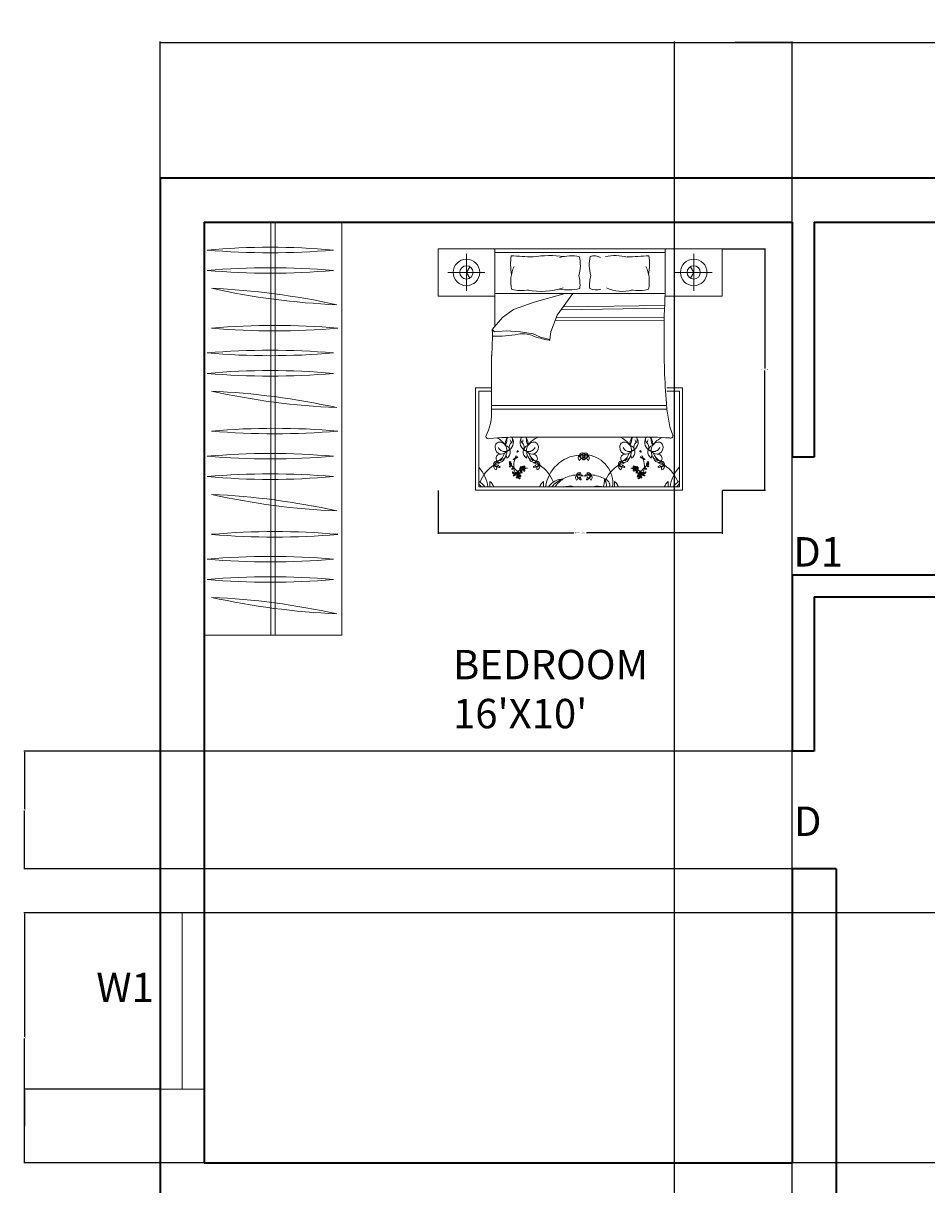
# Model space of a CAD drawing. Units: inches. Extents: x -4347 to -3836, y 955 to 1521.
# Tile 9 of 11: x -4347 to -4162, y 1284 to 1521. Entities that reach past the tile are written whole.
import ezdxf

# ---------------------------------------------------------------- set-up
doc = ezdxf.new("R2010")
doc.units = ezdxf.units.IN
doc.header["$MEASUREMENT"] = 0
for name, color, linetype, lineweight in [('A-ANNO-DIMS', 2, 'Continuous', 18), ('A-ANNO-TEXT', 7, 'Continuous', 18), ('A-AREA-IDEN', 7, 'Continuous', 18), ('A-FURN', 8, 'Continuous', 13), ('A-GLAZ', 4, 'Continuous', 18), ('A-WALL', 7, 'Continuous', 35)]:
    doc.layers.add(name, color=color, linetype=linetype, lineweight=lineweight)
doc.styles.get("Standard").update_dxf_attribs({"font": 'arial.ttf'})
doc.dimstyles.get("Standard").update_dxf_attribs({"dimtxt": 0.18, "dimasz": 0.18, "dimexe": 0.18, "dimexo": 0.0625, "dimgap": 0.09, "dimtad": 0, "dimtih": 1, "dimtoh": 1, "dimdec": 0, "dimzin": 0, "dimdsep": 46, "dimlunit": 3, "dimtxsty": 'Standard', "dimcen": 0.09, "dimadec": 0, "dimazin": 0, "dimtfac": 1, "dimtdec": 0, "dimtofl": 0, "dimtmove": 0, "dimatfit": 3, "dimfxl": 1, "dimtolj": 1, "dimtzin": 0, "dimarcsym": 0})

# ---------------------------------------------------------------- blocks, each defined once
blk = doc.blocks.new('*D1')
at = {"layer": 'A-ANNO-DIMS', "color": 0, "lineweight": -2, "transparency": 16777216}
for p, q in [((-4318.58, 1489.85), (-4318.58, 1517.61)), ((-4318.4, 1517.43), (-4135.47, 1517.43)), ((-3931.76, 1517.43), (-4114.69, 1517.43)), ((-3931.58, 1489.85), (-3931.58, 1517.61))]:
    blk.add_line(p, q, dxfattribs=at)
at = {"layer": 'A-ANNO-DIMS', "color": 0, "transparency": 16777216}
for points in [[(-4318.4, 1517.46), (-4318.4, 1517.4), (-4318.58, 1517.43)], [(-3931.76, 1517.46), (-3931.76, 1517.4), (-3931.58, 1517.43)]]:
    blk.add_solid(points, dxfattribs=at)
at = {"layer": 'Defpoints', "color": 0, "transparency": 16777216}
for p in [(-3931.58, 1517.43), (-4318.58, 1489.79), (-3931.58, 1489.79)]:
    blk.add_point(p, dxfattribs=at)
at = {"layer": 'A-ANNO-DIMS', "color": 0, "transparency": 16777216, "insert": (-4125.08, 1517.43), "char_height": 6, "attachment_point": 5}
blk.add_mtext('\\A1;32\'-3"', dxfattribs=at)
blk = doc.blocks.new('BED-DOUBLE-WITH-NIGHTSTANDS')
for p, q in [((0, 49.3), (57.97, 49.3)), ((5.8, 40.68), (5.8, 48.26)), ((11.59, 49.3), (11.59, 33.39)), ((46.38, 48.56), (11.59, 48.56)), ((52.18, 40.68), (52.18, 48.26)), ((9.59, 44.47), (2.01, 44.47)), ((48.39, 44.47), (55.96, 44.47)), ((11.59, 40.14), (46.38, 40.14)), ((15.42, 36.89), (19.65, 38.42)), ((19.65, 38.42), (25.97, 40.14)), ((27.52, 40.14), (24.34, 35.72)), ((13.19, 35.25), (15.42, 36.89)), ((24.34, 35.72), (23.05, 32.32)), ((46.2, 37.14), (25.15, 36.84)), ((46.22, 37.73), (25.58, 37.44)), ((11.08, 32.79), (13.19, 35.25)), ((46.17, 34.72), (23.93, 34.63)), ((46.17, 35.31), (24.16, 35.23)), ((11.55, 32.32), (11.08, 32.79)), ((13.89, 32.55), (11.55, 32.32)), ((16.83, 32.32), (13.89, 32.55)), ((19.41, 31.96), (16.83, 32.32)), ((20.94, 31.26), (19.41, 31.96)), ((22.82, 30.79), (20.94, 31.26)), ((23.05, 32.32), (22.82, 30.79)), ((7.65, 20.88), (10.93, 20.88)), ((7.65, 0), (7.65, 20.88)), ((10.93, 20.21), (8.32, 20.21)), ((8.32, 20.21), (8.32, 0.67)), ((49.25, 20.21), (46.69, 20.21)), ((46.7, 20.88), (49.92, 20.88)), ((49.25, 0.67), (49.25, 20.21)), ((49.92, 20.88), (49.92, 0)), ((46.64, 17.27), (10.93, 17.27)), ((46.7, 16.54), (10.93, 16.54)), ((40.76, 10.85), (17.22, 10.85)), ((14.04, 6.55), (13.91, 7.2)), ((18.09, 6.55), (18.22, 7.2)), ((39.48, 6.55), (39.35, 7.2)), ((43.53, 6.55), (43.66, 7.2)), ((8.32, 0.67), (49.25, 0.67)), ((49.92, 0), (7.65, 0))]:
    blk.add_line(p, q)
for points in [[(11.59, 39.64), (0, 39.64), (0, 49.3)], [(46.38, 49.3), (46.38, 39.64), (57.97, 39.64), (57.97, 49.3)], [(5.8, 44.47), (6.47, 45.64)], [(52.18, 44.47), (51.5, 45.64)], [(5.8, 44.47), (6.47, 43.3)], [(52.18, 44.47), (51.5, 43.3)]]:
    blk.add_lwpolyline(points)
for points in [[(14.92, 47.86, 0.074897), (15, 44.07, -0.472817)], [(28.72, 43.86, 0.14099), (28.83, 47.72, 0.235245)], [(31.19, 43.86, -0.14099), (31.08, 47.72, -0.235245)], [(43.05, 47.86, -0.074897), (42.98, 44.07, 0.472817)], [(10.95, 27.48, 0.001242), (10.93, 16.48, -0.127202), (9.76, 10.99)], [(46.63, 17.72, 0.056112), (47.05, 14.53, 0.095341), (47.86, 11.46)]]:
    blk.add_lwpolyline(points, format="xyb")
for centre, radius in [((5.8, 44.47), 2.71), ((5.8, 44.47), 1.35), ((52.18, 44.47), 2.71), ((52.18, 44.47), 1.35), ((16.42, 2.89), 0.148), ((17.39, 4.45), 0.148), ((40.18, 4.45), 0.148), ((41.15, 2.89), 0.148)]:
    blk.add_circle(centre, radius)
for centre, radius, start, end in [((46.88, 599.58), 552.65, 266.6852, 267.1498), ((22.87, 26.88), 21.03, 82.2196, 99.497), ((27.31, 37.51), 10.33, 81.5249, 103.96), ((31.87, 44.97), 2.87, 63.3437, 106.1026), ((36.17, 37.71), 10.19, 76.3427, 101.1841), ((11.09, 599.58), 552.65, 272.8502, 273.3148), ((22.31, 42.55), 7.47, 155.1316, 191.7583), ((35.66, 42.55), 7.47, 348.2417, 24.8684), ((21.88, 41.92), 7.1, 354.0129, 15.8293), ((38.03, 41.92), 7.1, 164.1707, 185.9871), ((16.99, 48.54), 7.77, 255.1039, 281.0369), ((21.08, 54.06), 13.48, 258.0397, 289.2615), ((26.54, 51.12), 10.22, 259.8617, 283.6238), ((32.26, 43.97), 3.07, 245.0183, 288.5407), ((37.63, 47.96), 7.38, 243.8761, 286.1746), ((40.98, 48.54), 7.77, 258.9631, 284.8961), ((150.31, 33.06), 104.17, 176.1, 180.9282), ((-42.08, 31.34), 53.18, 355.8294, 1.553), ((12.07, 53.32), 21.88, 267.4519, 281.3392), ((17.3, 27.24), 4.72, 66.2616, 101.3392), ((26.84, 52.7), 22.48, 250.1194, 259.3383), ((182.02, 29.27), 135.88, 179.1145, 184.8735), ((22.69, 30.74), 0.14, 268.8623, 19.7536), ((10.3, 11.03), 0.535, 183.98, 297.3412), ((16.53, -49.5), 60.35, 89.3433, 95.6887), ((12.63, 8.87), 0.979, 84.4856, 181.0538), ((10.07, 6.77), 4.39, 33.6671, 63.2997), ((12.33, 8.15), 1.74, 355.2933, 76.921), ((15.95, 9.38), 2.24, 145.785, 184.7304), ((11.68, 10.42), 2.4, 328.8218, 9.1554), ((14.66, 10.21), 0.698, 120.0293, 142.325), ((13.54, 9.8), 1.85, 289.2822, 29.1751), ((15.73, 8.81), 1.19, 131.5653, 195.1471), ((13.26, 9.46), 1.67, 7.436, 29.9149), ((14.36, 10.35), 0.867, 311.5653, 23.8354), ((14.66, 10.21), 0.698, 44.4517, 63.558), ((18.58, 9.8), 1.85, 150.8249, 250.7178), ((17.76, 10.35), 0.867, 156.1646, 228.4347), ((17.47, 10.21), 0.698, 113.229, 135.5483), ((16.4, 8.81), 1.19, 344.8529, 48.4347), ((18.86, 9.46), 1.67, 150.0851, 172.564), ((17.47, 10.21), 0.698, 37.675, 66.7144), ((16.17, 9.38), 2.24, 355.2696, 34.215), ((20.44, 10.42), 2.4, 169.7133, 211.1782), ((19.8, 8.15), 1.74, 103.079, 184.7067), ((22.05, 6.77), 4.39, 111.4941, 146.3329), ((19.5, 8.87), 0.979, 358.9462, 95.5144), ((38.07, 8.87), 0.979, 84.4856, 181.0538), ((35.52, 6.77), 4.39, 33.6671, 68.5059), ((37.77, 8.15), 1.74, 355.2933, 76.921), ((41.4, 9.38), 2.24, 145.785, 184.7304), ((37.13, 10.42), 2.4, 328.8218, 10.2867), ((40.1, 10.21), 0.698, 113.2856, 142.325), ((38.99, 9.8), 1.85, 289.2822, 29.1751), ((41.17, 8.81), 1.19, 131.5653, 195.1471), ((38.71, 9.46), 1.67, 7.436, 29.9149), ((40.1, 10.21), 0.698, 44.4517, 66.7144), ((39.81, 10.35), 0.867, 311.5653, 23.8354), ((42.53, -45.54), 56.41, 85.2402, 91.8035), ((44.03, 9.8), 1.85, 150.8249, 250.7178), ((43.21, 10.35), 0.867, 156.1646, 228.4347), ((42.91, 10.21), 0.698, 106.6343, 135.5483), ((41.84, 8.81), 1.19, 344.8529, 48.4347), ((44.31, 9.46), 1.67, 150.0851, 172.564), ((42.91, 10.21), 0.698, 37.675, 72.5814), ((41.62, 9.38), 2.24, 355.2696, 34.215), ((45.89, 10.42), 2.4, 169.249, 211.1782), ((45.24, 8.15), 1.74, 103.079, 184.7067), ((47.5, 6.77), 4.39, 113.6453, 146.3329), ((44.94, 8.87), 0.979, 358.9462, 95.5144), ((47.42, 11.17), 0.528, 246.5219, 33.8264), ((13.03, 8.73), 1.39, 174.9449, 262.8857), ((12.71, 6.5), 0.87, 80.264, 250.8688), ((13.57, 9.26), 1.35, 201.5819, 291.4221), ((10.99, 8.42), 2.74, 301.2614, 341.7045), ((12.79, 9.04), 1.68, 272.3591, 324.0401), ((10.96, 8.2), 3.11, 326.2883, 356.5076), ((13.32, 7.8), 1.44, 299.9085, 73.1337), ((15.95, 9.38), 2.24, 212.7011, 216.3445), ((14.23, 8.4), 0.36, 257.3041, 15.1471), ((20.25, 4.94), 4.8, 153.0032, 159.8941), ((16.23, 7.86), 0.112, 102.7051, 280.4384), ((16.22, 7.93), 0.182, 280.4384, 100.4136), ((18.81, 7.8), 1.44, 106.8663, 240.0915), ((17.89, 8.4), 0.36, 164.8529, 282.6959), ((16.17, 9.38), 2.24, 323.6555, 327.2989), ((19.34, 9.04), 1.68, 215.9599, 267.6409), ((18.55, 9.26), 1.35, 248.5779, 338.4181), ((21.17, 8.2), 3.11, 183.4924, 213.7117), ((21.14, 8.42), 2.74, 198.2955, 238.7386), ((19.1, 8.73), 1.39, 277.1143, 5.0551), ((19.41, 6.5), 0.87, 289.1312, 99.736), ((29.44, -0.35), 7.57, 94.4623, 172.255), ((29.47, 6.63), 0.84, 137.7873, 219.1145), ((28.52, 6.66), 0.632, 298.5391, 58.3627), ((29.45, 7.02), 0.628, 63.0274, 163.8037), ((28.82, 8.49), 1.29, 271.4585, 315.3727), ((29.34, 6.11), 1.2, 45.5411, 114.3101), ((30.43, 12.25), 5.3, 252.593, 267.2582), ((29.47, 7.17), 0.619, 177.7585, 283.852), ((30.66, 7.82), 1.91, 198.9159, 238.011), ((30.16, 6.11), 1.2, 65.6899, 134.4589), ((29.07, 12.25), 5.3, 272.7418, 287.407), ((30.05, 7.02), 0.628, 16.1963, 116.9726), ((30.69, 8.49), 1.29, 224.6273, 268.5415), ((28.84, 7.82), 1.91, 301.989, 341.0841), ((30.03, 7.17), 0.619, 256.148, 2.2415), ((30.99, 6.66), 0.632, 121.6373, 241.4609), ((30.03, 6.63), 0.84, 320.8855, 42.2127), ((29.82, 1.4), 5.86, 352.8636, 81.8197), ((38.47, 8.73), 1.39, 174.9449, 262.8857), ((38.16, 6.5), 0.87, 80.264, 250.8688), ((39.02, 9.26), 1.35, 201.5819, 291.4221), ((36.43, 8.42), 2.74, 301.2614, 341.7045), ((38.23, 9.04), 1.68, 272.3591, 324.0401), ((36.4, 8.2), 3.11, 326.2883, 356.5076), ((38.76, 7.8), 1.44, 299.9085, 73.1337), ((41.4, 9.38), 2.24, 212.7011, 216.3445), ((39.68, 8.4), 0.36, 257.3041, 15.1471), ((41.35, 7.93), 0.182, 79.5864, 259.5616), ((41.34, 7.86), 0.112, 259.5616, 77.2949), ((37.32, 4.94), 4.8, 20.1059, 26.9968), ((44.25, 7.8), 1.44, 106.8663, 240.0915), ((43.34, 8.4), 0.36, 164.8529, 282.6959), ((41.62, 9.38), 2.24, 323.6555, 327.2989), ((44.78, 9.04), 1.68, 215.9599, 267.6409), ((44, 9.26), 1.35, 248.5779, 338.4181), ((46.61, 8.2), 3.11, 183.4924, 213.7117), ((46.58, 8.42), 2.74, 198.2955, 238.7386), ((44.54, 8.73), 1.39, 277.1143, 5.0551), ((44.86, 6.5), 0.87, 289.1312, 99.736), ((15.64, -1.1), 7.57, 124.3865, 158.5908), ((12.18, 4.97), 0.84, 167.7115, 249.0387), ((11.97, 5.3), 0.628, 92.9516, 193.728), ((10.69, 6.25), 1.29, 301.3827, 345.2969), ((12.34, 4.45), 1.2, 75.4653, 144.2343), ((10.22, 10.32), 5.3, 282.5173, 297.1824), ((11.35, 4.52), 0.632, 328.4633, 88.2869), ((12.62, 6.59), 1.91, 228.8402, 267.9352), ((11.91, 5.44), 0.619, 207.6827, 313.7762), ((12.53, 5.56), 0.533, 63.9755, 143.2681), ((12.28, 5.05), 0.0819, 313.7762, 249.7183), ((12.5, 6.76), 1.09, 265.969, 344.3045), ((12.55, 4.82), 0.0457, 101.4834, 217.9409), ((12.56, 4.77), 0.094, 267.9352, 101.4834), ((13.67, 5.32), 1.16, 96.1662, 141.5825), ((14.73, 5.55), 0.246, 101.5637, 142.6358), ((14.52, 5.33), 0.148, 273.2768, 86.7232), ((14.73, 5.05), 0.244, 217.7621, 259.0403), ((14.7, 5.47), 0.141, 91.1081, 181.8675), ((14.99, 5.38), 0.448, 203.4276, 227.6104), ((14.53, 5.75), 0.355, 288.7263, 352.5032), ((14.85, 5.18), 0.305, 80.3487, 133.6538), ((14.79, 5.43), 0.242, 229.7889, 317.6792), ((14.52, 4.92), 0.343, 355.053, 68.3618), ((14.79, 4.86), 0.483, 83.0852, 105.7171), ((14.77, 5.73), 0.114, 345.2356, 144.9248), ((14.75, 4.9), 0.113, 232.4737, 355.053), ((11.44, 0.86), 5.5, 43.1541, 52.0459), ((14.88, 5.36), 0.127, 317.6792, 80.3487), ((15.59, 6.13), 0.304, 101.3256, 154.4621), ((15.15, 7.16), 0.916, 280.2588, 300.656), ((15.36, 7.9), 1.63, 268.3264, 277.1302), ((20.25, 4.94), 4.8, 163.5842, 183.8277), ((14.95, 7.16), 0.931, 308.2101, 316.3071), ((15.52, 6.55), 0.278, 278.3432, 4.2869), ((15.37, 6.79), 0.486, 300.656, 332.6341), ((15.74, 6.47), 0.118, 55.7657, 157.4417), ((15.92, 6.58), 0.118, 84.3784, 186.0543), ((15.81, 7.06), 0.486, 269.1859, 301.164), ((15.95, 6.81), 0.278, 237.5332, 323.4768), ((15.68, 7.6), 0.931, 285.5129, 293.6099), ((15.59, 7.42), 0.916, 301.164, 321.5612), ((16.29, 6.55), 0.304, 87.3579, 140.4944), ((14.84, 7.58), 1.63, 324.6898, 333.4936), ((16.26, 4.67), 0.673, 304.5369, 16.3699), ((17.19, 4.48), 0.476, 127.3105, 187.9252), ((16.54, 4.53), 0.489, 355.0106, 41.658), ((17.22, 4.65), 0.201, 126.1046, 271.4281), ((17.2, 4.71), 0.145, 353.7526, 131.7054), ((17.59, 4.68), 0.246, 101.5637, 176.365), ((17.39, 4.87), 0.355, 288.7263, 352.5032), ((17.63, 4.85), 0.114, 345.2356, 144.9248), ((18.45, 5.32), 1.16, 38.4175, 83.8338), ((19.62, 6.76), 1.09, 195.6955, 274.031), ((19.59, 5.56), 0.533, 36.7319, 116.0245), ((19.57, 4.77), 0.094, 78.5166, 272.0648), ((19.79, 4.45), 1.2, 35.7657, 104.5347), ((21.91, 10.32), 5.3, 242.8176, 257.4827), ((19.5, 6.59), 1.91, 272.0648, 311.1598), ((19.58, 4.82), 0.0457, 322.0591, 78.5166), ((20.21, 5.44), 0.619, 226.2238, 332.3173), ((19.85, 5.08), 0.0494, 290.2667, 226.2271), ((20.78, 4.52), 0.632, 91.7131, 211.5367), ((20.15, 5.3), 0.628, 346.272, 87.0484), ((21.43, 6.25), 1.29, 194.7031, 238.6173), ((19.94, 4.97), 0.84, 290.9613, 12.2885), ((16.49, -1.1), 7.57, 21.4092, 55.6135), ((29.6, 6.65), 0.0819, 283.852, 219.9245), ((29.7, 6.28), 0.094, 238.011, 71.5592), ((29.71, 6.32), 0.0457, 71.5592, 188.0167), ((29.81, 6.28), 0.094, 108.4408, 301.989), ((29.79, 6.32), 0.0457, 351.9833, 108.4408), ((29.9, 6.68), 0.0494, 320.1909, 256.0209), ((41.08, -1.1), 7.57, 124.3865, 158.5908), ((37.42, 5.3), 0.628, 92.9516, 193.728), ((37.63, 4.97), 0.84, 167.7115, 249.0387), ((36.13, 6.25), 1.29, 301.3827, 345.2969), ((37.78, 4.45), 1.2, 75.4653, 144.2343), ((35.66, 10.32), 5.3, 282.5173, 297.1824), ((37.36, 5.44), 0.619, 207.6827, 313.7762), ((38.07, 6.59), 1.91, 228.8402, 267.9352), ((36.79, 4.52), 0.632, 328.4633, 88.2869), ((37.98, 5.56), 0.533, 63.9755, 143.2681), ((37.73, 5.05), 0.0819, 313.7762, 249.7183), ((37.95, 6.76), 1.09, 265.969, 344.3045), ((37.99, 4.82), 0.0457, 101.4834, 217.9409), ((38, 4.77), 0.094, 267.9352, 101.4834), ((39.12, 5.32), 1.16, 96.1662, 141.5825), ((39.94, 4.85), 0.114, 35.0752, 194.7644), ((40.18, 4.87), 0.355, 187.4968, 251.2737), ((39.98, 4.68), 0.246, 3.635, 78.4363), ((40.37, 4.71), 0.145, 48.2946, 186.2474), ((40.35, 4.65), 0.201, 268.5719, 53.8954), ((41.03, 4.53), 0.489, 138.342, 184.9894), ((41.31, 4.67), 0.673, 163.6301, 235.4631), ((40.38, 4.48), 0.476, 352.0748, 52.6895), ((41.98, 7.42), 0.916, 218.4388, 238.836), ((41.28, 6.55), 0.304, 39.5056, 92.6421), ((42.73, 7.58), 1.63, 206.5064, 215.3102), ((41.62, 6.81), 0.278, 216.5232, 302.4668), ((41.89, 7.6), 0.931, 246.3901, 254.4871), ((41.76, 7.06), 0.486, 238.836, 270.8141), ((41.65, 6.58), 0.118, 353.9457, 95.6216), ((41.83, 6.47), 0.118, 22.5583, 124.2343), ((42.05, 6.55), 0.278, 175.7131, 261.6568), ((42.2, 6.79), 0.486, 207.3659, 239.344), ((37.32, 4.94), 4.8, 356.1723, 16.4158), ((42.62, 7.16), 0.931, 223.6929, 231.7899), ((42.42, 7.16), 0.916, 239.344, 259.7412), ((42.21, 7.9), 1.63, 262.8698, 271.6736), ((41.98, 6.13), 0.304, 25.5379, 78.6744), ((46.13, 0.86), 5.5, 127.9541, 136.8459), ((42.69, 5.36), 0.127, 99.6513, 222.3208), ((42.78, 5.43), 0.242, 222.3208, 310.2111), ((42.72, 5.18), 0.305, 46.3462, 99.6513), ((42.8, 5.73), 0.114, 35.0752, 194.7644), ((43.04, 5.75), 0.355, 187.4968, 251.2737), ((43.05, 4.92), 0.343, 111.6382, 184.947), ((42.82, 4.9), 0.113, 184.947, 307.5263), ((42.78, 4.86), 0.483, 74.2829, 96.9148), ((42.87, 5.47), 0.141, 358.1325, 88.8919), ((42.58, 5.38), 0.448, 312.3896, 336.5724), ((42.84, 5.55), 0.246, 37.3642, 78.4363), ((42.84, 5.05), 0.244, 280.9597, 322.2379), ((43.05, 5.33), 0.148, 93.2768, 266.7232), ((45.07, 6.76), 1.09, 195.6955, 274.031), ((43.9, 5.32), 1.16, 38.4175, 83.8338), ((45.04, 5.56), 0.533, 36.7319, 116.0245), ((45.01, 4.77), 0.094, 78.5166, 272.0648), ((45.23, 4.45), 1.2, 35.7657, 104.5347), ((47.35, 10.32), 5.3, 242.8176, 257.4827), ((44.95, 6.59), 1.91, 272.0648, 311.1598), ((45.02, 4.82), 0.0457, 322.0591, 78.5166), ((45.66, 5.44), 0.619, 226.2238, 332.3173), ((45.29, 5.08), 0.0494, 290.2667, 226.2271), ((46.22, 4.52), 0.632, 91.7131, 211.5367), ((46.88, 6.25), 1.29, 194.7031, 238.6173), ((45.6, 5.3), 0.628, 346.272, 87.0484), ((45.39, 4.97), 0.84, 290.9613, 12.2885), ((41.93, -1.1), 7.57, 21.4092, 55.6135), ((2.69, -0.35), 7.57, 7.745, 41.8856), ((15.24, 4.18), 0.304, 101.3256, 154.4621), ((14.81, 5.21), 0.916, 280.2588, 300.656), ((15.02, 5.95), 1.63, 268.3264, 277.1302), ((14.61, 5.21), 0.931, 308.2101, 316.3071), ((15.35, 3.65), 0.165, 146.8636, 236.9021), ((17.67, 7.28), 4.31, 235.1882, 238.8844), ((15.63, 3.89), 0.446, 199.4799, 267.6828), ((15.18, 4.6), 0.278, 278.3432, 4.2869), ((15.58, 3.72), 0.384, 212.8155, 277.3992), ((15.03, 4.84), 0.486, 300.656, 332.6341), ((15.39, 4.52), 0.118, 55.7657, 157.4417), ((15.36, 3.46), 0.446, 266.9701, 338.2913), ((13, 6.64), 4.31, 302.6784, 306.3746), ((15.47, 3.11), 0.165, 214.3538, 304.3923), ((15.53, 3.73), 0.171, 238.8844, 314.2646), ((17.86, 4.82), 2.41, 184.756, 209.2041), ((21.32, 9.95), 7.92, 222.2412, 232.1744), ((15.49, 3.35), 0.384, 280.3057, 17.1958), ((15.46, 3.31), 0.171, 306.3746, 21.7548), ((15.74, 3.42), 0.129, 19.3605, 201.7548), ((15.74, 3.52), 0.129, 311.8703, 134.2646), ((18.16, 2.34), 2.57, 153.7819, 158.2913), ((16.11, 4.1), 0.673, 247.2305, 319.0635), ((15.89, 3.87), 0.396, 264.4544, 310.6188), ((17.86, 4.82), 2.41, 214.0033, 222.4917), ((16.18, 3.72), 0.409, 218.3208, 298.8162), ((18.1, 1.62), 2.89, 120.544, 139.818), ((16.11, 2.62), 0.146, 148.0499, 225.6268), ((16.38, 2.45), 0.465, 104.7558, 148.0499), ((16.12, 2.78), 0.291, 247.4086, 351.4386), ((16.26, 3.1), 0.201, 126.1046, 271.4281), ((16.24, 3.15), 0.145, 353.7526, 131.7054), ((16.46, 3.21), 0.476, 70.0041, 130.6188), ((16.2, 2.77), 0.0978, 262.906, 7.132), ((16.1, 2.98), 0.203, 0.0645, 61.1507), ((16.15, 3.15), 0.232, 311.8413, 355.7877), ((16.15, 3.79), 0.489, 297.7043, 344.3516), ((16.62, 3.12), 0.246, 101.5637, 176.365), ((16.62, 2.62), 0.244, 151.2196, 259.0403), ((16.59, 3.03), 0.141, 91.1081, 181.8675), ((16.88, 2.94), 0.448, 203.4276, 227.6104), ((16.74, 2.75), 0.305, 80.3487, 133.6538), ((16.69, 3), 0.242, 229.7889, 317.6792), ((16.43, 3.31), 0.355, 288.7263, 352.5032), ((16.42, 2.49), 0.343, 355.053, 68.3618), ((16.68, 2.43), 0.483, 83.0852, 105.7171), ((16.67, 3.3), 0.114, 345.2356, 144.9248), ((16.64, 2.47), 0.113, 232.4737, 355.053), ((16.62, 4.52), 0.409, 272.8499, 356.1226), ((16.33, 4.36), 0.396, 321.7607, 7.9252), ((16.41, 3.79), 0.396, 8.7227, 54.8872), ((16.43, 3.47), 0.673, 0.278, 72.111), ((16.73, 3.72), 0.409, 20.5253, 88.5375), ((16.77, 2.92), 0.127, 317.6792, 80.3487), ((17.27, 3.92), 0.476, 188.7227, 249.3375), ((17.08, 4.17), 0.146, 148.0499, 225.6268), ((18.1, 1.62), 2.89, 113.0501, 113.8477), ((17.35, 4), 0.465, 104.7558, 148.0499), ((17.09, 4.34), 0.291, 247.4086, 351.4386), ((16.66, 3.68), 0.489, 334.9899, 21.6373), ((17.06, 4.54), 0.203, 0.0645, 61.1507), ((17.17, 4.32), 0.0978, 262.906, 7.132), ((17.11, 4.71), 0.232, 311.8413, 355.7877), ((17.59, 4.18), 0.244, 151.2196, 259.0403), ((17.56, 4.59), 0.141, 91.1081, 181.8675), ((17.85, 4.5), 0.448, 203.4276, 227.6104), ((17.71, 4.3), 0.305, 80.3487, 133.6538), ((17.65, 4.56), 0.242, 229.7889, 317.6792), ((17.38, 4.05), 0.343, 355.053, 68.3618), ((17.65, 3.99), 0.483, 83.0852, 105.7171), ((17.61, 4.03), 0.113, 232.4737, 355.053), ((17.74, 4.48), 0.127, 317.6792, 80.3487), ((18.1, 1.62), 2.89, 87.1071, 94.7585), ((28.86, -4.4), 7.57, 94.4623, 117.4146), ((28.89, 2.58), 0.84, 137.7873, 219.1145), ((27.94, 2.61), 0.632, 298.5391, 58.3627), ((28.87, 2.97), 0.628, 63.0274, 163.8037), ((28.24, 4.44), 1.29, 271.4585, 315.3727), ((28.76, 2.05), 1.2, 45.5411, 114.3101), ((30.08, 3.76), 1.91, 198.9159, 238.011), ((29.85, 8.2), 5.3, 252.593, 267.2582), ((28.89, 3.12), 0.619, 177.7585, 283.852), ((29.02, 2.6), 0.0819, 283.852, 219.9245), ((30.74, 2.05), 1.2, 65.6899, 134.4589), ((29.65, 8.2), 5.3, 272.7418, 287.407), ((30.63, 2.97), 0.628, 16.1963, 116.9726), ((31.27, 4.44), 1.29, 224.6273, 268.5415), ((30.48, 2.63), 0.0494, 320.1909, 256.0209), ((29.42, 3.76), 1.91, 301.989, 341.0841), ((30.61, 3.12), 0.619, 256.148, 2.2415), ((31.56, 2.61), 0.632, 121.6373, 241.4609), ((30.61, 2.58), 0.84, 320.8855, 42.2127), ((30.64, -4.4), 7.57, 62.5854, 85.5377), ((39.47, 1.62), 2.89, 85.2415, 92.8929), ((39.83, 4.48), 0.127, 99.6513, 222.3208), ((39.92, 4.56), 0.242, 222.3208, 310.2111), ((39.86, 4.3), 0.305, 46.3462, 99.6513), ((40.19, 4.05), 0.343, 111.6382, 184.947), ((39.96, 4.03), 0.113, 184.947, 307.5263), ((39.92, 3.99), 0.483, 74.2829, 96.9148), ((40.01, 4.59), 0.141, 358.1325, 88.8919), ((39.72, 4.5), 0.448, 312.3896, 336.5724), ((39.98, 4.18), 0.244, 280.9597, 28.7804), ((40.48, 4.34), 0.291, 188.5614, 292.5914), ((40.46, 4.71), 0.232, 184.2123, 228.1587), ((40.5, 4.54), 0.203, 118.8493, 179.9355), ((40.4, 4.32), 0.0978, 172.868, 277.094), ((40.22, 4), 0.465, 31.9501, 75.2442), ((40.91, 3.68), 0.489, 158.3627, 205.0101), ((40.84, 3.72), 0.409, 91.4625, 159.4747), ((41.14, 3.47), 0.673, 107.889, 179.722), ((40.3, 3.92), 0.476, 290.6625, 351.2773), ((40.95, 4.52), 0.409, 183.8774, 267.1501), ((39.47, 1.62), 2.89, 66.1523, 66.9499), ((40.49, 4.17), 0.146, 314.3732, 31.9501), ((40.8, 2.92), 0.127, 99.6513, 222.3208), ((40.88, 3), 0.242, 222.3208, 310.2111), ((41.16, 3.79), 0.396, 125.1128, 171.2773), ((40.83, 2.75), 0.305, 46.3462, 99.6513), ((40.9, 3.3), 0.114, 35.0752, 194.7644), ((41.14, 3.31), 0.355, 187.4968, 251.2737), ((41.15, 2.49), 0.343, 111.6382, 184.947), ((40.93, 2.47), 0.113, 184.947, 307.5263), ((40.89, 2.43), 0.483, 74.2829, 96.9148), ((41.24, 4.36), 0.396, 172.0748, 218.2393), ((39.47, 1.62), 2.89, 40.182, 59.456), ((41.11, 3.21), 0.476, 49.3812, 109.9959), ((41.46, 4.1), 0.673, 220.9365, 292.7695), ((41.42, 3.79), 0.489, 195.6484, 242.2957), ((40.98, 3.03), 0.141, 358.1325, 88.8919), ((40.95, 3.12), 0.246, 3.635, 78.4363), ((40.68, 2.94), 0.448, 312.3896, 336.5724), ((40.95, 2.62), 0.244, 280.9597, 28.7804), ((36.25, 9.95), 7.92, 307.8256, 317.7588), ((41.45, 2.78), 0.291, 188.5614, 292.5914), ((41.39, 3.72), 0.409, 241.1838, 321.6792), ((41.33, 3.15), 0.145, 48.2946, 186.2474), ((41.42, 3.15), 0.232, 184.2123, 228.1587), ((41.47, 2.98), 0.203, 118.8493, 179.9355), ((41.37, 2.77), 0.0978, 172.868, 277.094), ((41.31, 3.1), 0.201, 268.5719, 53.8954), ((41.19, 2.45), 0.465, 31.9501, 75.2442), ((41.68, 3.87), 0.396, 229.3812, 275.5456), ((39.71, 4.82), 2.41, 317.5083, 325.9967), ((41.46, 2.62), 0.146, 314.3732, 31.9501), ((42.08, 3.35), 0.384, 162.8042, 259.6943), ((41.83, 3.52), 0.129, 45.7354, 228.1297), ((41.83, 3.42), 0.129, 338.2452, 160.6395), ((39.41, 2.34), 2.57, 21.7087, 26.2181), ((42.21, 3.46), 0.446, 201.7087, 273.0299), ((39.71, 4.82), 2.41, 330.7959, 355.244), ((42.04, 3.73), 0.171, 225.7354, 301.1156), ((41.99, 3.72), 0.384, 262.6008, 327.1845), ((42.11, 3.31), 0.171, 158.2452, 233.6254), ((41.94, 3.89), 0.446, 272.3172, 340.5201), ((44.57, 6.64), 4.31, 233.6254, 237.3216), ((42.1, 3.11), 0.165, 235.6077, 325.6462), ((42.18, 4.52), 0.118, 22.5583, 124.2343), ((42.39, 4.6), 0.278, 175.7131, 261.6568), ((42.54, 4.84), 0.486, 207.3659, 239.344), ((39.9, 7.28), 4.31, 301.1156, 304.8118), ((42.96, 5.21), 0.931, 223.6929, 231.7899), ((42.76, 5.21), 0.916, 239.344, 259.7412), ((42.22, 3.65), 0.165, 303.0979, 33.1364), ((42.55, 5.95), 1.63, 262.8698, 271.6736), ((42.33, 4.18), 0.304, 25.5379, 78.6744), ((54.88, -0.35), 7.57, 138.1144, 172.255), ((6.49, -1.36), 3.69, 33.4617, 60.1116), ((5.16, -2.05), 4.6, 36.3036, 46.4814), ((8.55, -0.51), 3.08, 22.5547, 48.9546), ((0.12, 1.15), 10.47, 357.4081, 3.6519), ((23.57, -0.51), 3.08, 131.0454, 157.4453), ((32.01, 1.15), 10.47, 176.3481, 182.5919), ((25.64, -1.36), 3.69, 91.272, 146.5383), ((26.97, -2.05), 4.6, 107.8504, 143.6964), ((29.38, -3.34), 6.84, 124.0123, 144.053), ((26.74, -3.31), 4.16, 73.5431, 107.0202), ((28.39, -5.45), 6.16, 94.3787, 95.6357), ((31.63, -9.67), 11, 109.7217, 109.9028), ((29.12, 2.22), 0.094, 238.011, 71.5592), ((29.13, 2.27), 0.0457, 71.5592, 188.0167), ((30.39, 2.22), 0.094, 108.4408, 301.989), ((30.37, 2.27), 0.0457, 351.9833, 108.4408), ((32.76, -3.31), 4.16, 72.9798, 106.4569), ((31.11, -5.45), 6.16, 84.3643, 85.6213), ((27.87, -9.67), 11, 70.0972, 70.2783), ((30.58, 1.93), 3.39, 338.117, 6.6195), ((33.69, 0.99), 1.36, 346.3898, 79.0739), ((32.67, 1.18), 1.72, 342.8609, 41.9049), ((25.56, 1.15), 10.47, 357.4081, 3.6519), ((34, -0.51), 3.08, 22.5547, 48.9546), ((49.02, -0.51), 3.08, 131.0454, 157.4453), ((57.45, 1.15), 10.47, 176.3481, 182.5919), ((51.08, -1.36), 3.69, 119.8884, 146.5383), ((52.41, -2.05), 4.6, 133.5186, 143.6964)]:
    blk.add_arc(centre, radius, start, end)
blk = doc.blocks.new('WARDROBE-LONG')
for p, q in [((0, 0), (0, 84.3)), ((28.1, 84.3), (0, 84.3)), ((13.58, 0), (13.58, 84.3)), ((14.52, 0), (14.52, 84.3)), ((28.1, 0), (28.1, 84.3)), ((28.1, 0), (0, 0))]:
    blk.add_line(p, q)
for centre, start, end in [((13.49, -68.71), 85.0028, 94.9972), ((13.49, 225.88), 265.0028, 274.9972), ((13.49, -72.88), 85.0028, 94.9972), ((13.49, 221.72), 265.0028, 274.9972), ((33.49, 215.14), 257.508, 267.5023), ((-4.93, -76.94), 77.508, 87.5023), ((14.4, -84.65), 85.0028, 94.9972), ((14.4, 209.94), 265.0028, 274.9972), ((13.49, -89.72), 85.0028, 94.9972), ((13.49, 204.88), 265.0028, 274.9972), ((13.49, -93.88), 85.0028, 94.9972), ((13.49, 200.71), 265.0028, 274.9972), ((33.49, 194.14), 257.508, 267.5023), ((-4.93, -97.94), 77.508, 87.5023), ((14.4, -105.66), 85.0028, 94.9972), ((14.4, 188.94), 265.0028, 274.9972), ((13.49, -110.8), 85.0028, 94.9972), ((13.49, 183.8), 265.0028, 274.9972), ((13.49, -114.96), 85.0028, 94.9972), ((13.49, 179.63), 265.0028, 274.9972), ((-4.93, -119.02), 77.508, 87.5023), ((33.49, 173.05), 257.508, 267.5023), ((14.4, -126.74), 85.0028, 94.9972), ((14.4, 167.85), 265.0028, 274.9972), ((13.49, -131.8), 85.0028, 94.9972), ((13.49, 162.79), 265.0028, 274.9972), ((13.49, -135.96), 85.0028, 94.9972), ((13.49, 158.63), 265.0028, 274.9972), ((-4.93, -140.03), 77.508, 87.5023), ((33.49, 152.05), 257.508, 267.5023)]:
    blk.add_arc(centre, 147.86, start, end)
blk = doc.blocks.new('GLAZ-36IN')
for p, q in [((0, 0), (0, 36)), ((0, 36), (9, 36)), ((4.5, 36), (4.5, 0)), ((9, 36), (9, 0)), ((9, 0), (0, 0))]:
    blk.add_line(p, q)
blk = doc.blocks.new('*D14')
at = {"layer": 'A-ANNO-DIMS', "color": 0, "lineweight": -2, "transparency": 16777216}
for p, q in [((-4261.86, 1425.98), (-4261.86, 1417.16)), ((-4203.88, 1425.98), (-4203.88, 1417.16)), ((-4261.68, 1417.34), (-4234.15, 1417.34)), ((-4204.06, 1417.34), (-4231.59, 1417.34))]:
    blk.add_line(p, q, dxfattribs=at)
at = {"layer": 'A-ANNO-DIMS', "color": 0, "transparency": 16777216}
for points in [[(-4261.68, 1417.37), (-4261.68, 1417.31), (-4261.86, 1417.34)], [(-4204.06, 1417.37), (-4204.06, 1417.31), (-4203.88, 1417.34)]]:
    blk.add_solid(points, dxfattribs=at)
at = {"layer": 'Defpoints', "color": 0, "transparency": 16777216}
for p in [(-4261.86, 1426.04), (-4203.88, 1426.04), (-4203.88, 1417.34)]:
    blk.add_point(p, dxfattribs=at)
at = {"layer": 'A-ANNO-DIMS', "color": 0, "transparency": 16777216, "insert": (-4232.87, 1417.34), "char_height": 0.18, "attachment_point": 5}
blk.add_mtext('\\A1;BED SET 4\'-10" TYP.', dxfattribs=at)
blk = doc.blocks.new('*D15')
at = {"layer": 'A-ANNO-DIMS', "color": 0, "lineweight": -2, "transparency": 16777216}
for p, q in [((-4203.82, 1475.34), (-4195.01, 1475.34)), ((-4195.19, 1475.16), (-4195.19, 1450.87)), ((-4195.19, 1426.22), (-4195.19, 1450.51)), ((-4203.82, 1426.04), (-4195.01, 1426.04))]:
    blk.add_line(p, q, dxfattribs=at)
at = {"layer": 'A-ANNO-DIMS', "color": 0, "transparency": 16777216}
for points in [[(-4195.22, 1475.16), (-4195.16, 1475.16), (-4195.19, 1475.34)], [(-4195.22, 1426.22), (-4195.16, 1426.22), (-4195.19, 1426.04)]]:
    blk.add_solid(points, dxfattribs=at)
at = {"layer": 'Defpoints', "color": 0, "transparency": 16777216}
for p in [(-4203.88, 1475.34), (-4195.19, 1475.34), (-4203.88, 1426.04)]:
    blk.add_point(p, dxfattribs=at)
at = {"layer": 'A-ANNO-DIMS', "color": 0, "transparency": 16777216, "insert": (-4195.19, 1450.69), "char_height": 0.18, "attachment_point": 5}
blk.add_mtext('\\A1;4\'-1 1/2" TYP.', dxfattribs=at)
blk = doc.blocks.new('*D43')
at = {"layer": 'A-ANNO-DIMS', "color": 0, "lineweight": -2, "transparency": 16777216}
for p, q in [((-4318.64, 1303.77), (-4346.41, 1303.77)), ((-4346.23, 1303.59), (-4346.23, 1296.46)), ((-4346.23, 1288.97), (-4346.23, 1296.1)), ((-4309.64, 1288.79), (-4346.41, 1288.79))]:
    blk.add_line(p, q, dxfattribs=at)
at = {"layer": 'A-ANNO-DIMS', "color": 0, "transparency": 16777216}
for points in [[(-4346.26, 1303.59), (-4346.2, 1303.59), (-4346.23, 1303.77)], [(-4346.26, 1288.97), (-4346.2, 1288.97), (-4346.23, 1288.79)]]:
    blk.add_solid(points, dxfattribs=at)
at = {"layer": 'Defpoints', "color": 0, "transparency": 16777216}
for p in [(-4346.23, 1303.77), (-4318.58, 1303.77), (-4309.58, 1288.79)]:
    blk.add_point(p, dxfattribs=at)
at = {"layer": 'A-ANNO-DIMS', "color": 0, "transparency": 16777216, "insert": (-4346.23, 1296.28), "char_height": 0.18, "attachment_point": 5}
blk.add_mtext('\\A1;1\'-3"', dxfattribs=at)
blk = doc.blocks.new('*D48')
at = {"layer": 'A-ANNO-DIMS', "color": 0, "lineweight": -2, "transparency": 16777216}
for p, q in [((-4120.64, 1339.79), (-4346.41, 1339.79)), ((-4346.23, 1339.61), (-4346.23, 1314.47)), ((-4346.23, 1288.97), (-4346.23, 1314.11)), ((-4120.64, 1288.79), (-4346.41, 1288.79))]:
    blk.add_line(p, q, dxfattribs=at)
at = {"layer": 'A-ANNO-DIMS', "color": 0, "transparency": 16777216}
for points in [[(-4346.26, 1339.61), (-4346.2, 1339.61), (-4346.23, 1339.79)], [(-4346.26, 1288.97), (-4346.2, 1288.97), (-4346.23, 1288.79)]]:
    blk.add_solid(points, dxfattribs=at)
at = {"layer": 'Defpoints', "color": 0, "transparency": 16777216}
for p in [(-4346.23, 1339.79), (-4120.58, 1339.79), (-4120.58, 1288.79)]:
    blk.add_point(p, dxfattribs=at)
at = {"layer": 'A-ANNO-DIMS', "color": 0, "transparency": 16777216, "insert": (-4346.23, 1314.29), "char_height": 0.18, "attachment_point": 5}
blk.add_mtext('\\A1;4\'-3"', dxfattribs=at)
blk = doc.blocks.new('*D58')
at = {"layer": 'A-ANNO-DIMS', "color": 0, "lineweight": -2, "transparency": 16777216}
for p, q in [((-4213.58, 1159.85), (-4213.58, 1517.62)), ((-4213.4, 1517.44), (-4201.91, 1517.44)), ((-4189.76, 1517.44), (-4201.25, 1517.44)), ((-4189.58, 1159.85), (-4189.58, 1517.62))]:
    blk.add_line(p, q, dxfattribs=at)
at = {"layer": 'A-ANNO-DIMS', "color": 0, "transparency": 16777216}
for points in [[(-4213.4, 1517.47), (-4213.4, 1517.41), (-4213.58, 1517.44)], [(-4189.76, 1517.47), (-4189.76, 1517.41), (-4189.58, 1517.44)]]:
    blk.add_solid(points, dxfattribs=at)
at = {"layer": 'Defpoints', "color": 0, "transparency": 16777216}
for p in [(-4189.58, 1517.44), (-4213.58, 1159.79), (-4189.58, 1159.79)]:
    blk.add_point(p, dxfattribs=at)
at = {"layer": 'A-ANNO-DIMS', "color": 0, "transparency": 16777216, "insert": (-4201.58, 1517.44), "char_height": 0.18, "attachment_point": 5}
blk.add_mtext('\\A1;2\'-0"', dxfattribs=at)
blk = doc.blocks.new('*D60')
at = {"layer": 'A-ANNO-DIMS', "color": 0, "lineweight": -2, "transparency": 16777216}
for p, q in [((-4189.64, 1372.79), (-4346.41, 1372.79)), ((-4346.23, 1372.61), (-4346.23, 1360.97)), ((-4346.23, 1348.97), (-4346.23, 1360.61)), ((-4189.64, 1348.79), (-4346.41, 1348.79))]:
    blk.add_line(p, q, dxfattribs=at)
at = {"layer": 'A-ANNO-DIMS', "color": 0, "transparency": 16777216}
for points in [[(-4346.26, 1372.61), (-4346.2, 1372.61), (-4346.23, 1372.79)], [(-4346.26, 1348.97), (-4346.2, 1348.97), (-4346.23, 1348.79)]]:
    blk.add_solid(points, dxfattribs=at)
at = {"layer": 'Defpoints', "color": 0, "transparency": 16777216}
for p in [(-4346.23, 1372.79), (-4189.58, 1372.79), (-4189.58, 1348.79)]:
    blk.add_point(p, dxfattribs=at)
at = {"layer": 'A-ANNO-DIMS', "color": 0, "transparency": 16777216, "insert": (-4346.23, 1360.79), "char_height": 0.18, "attachment_point": 5}
blk.add_mtext('\\A1;2\'-0"', dxfattribs=at)

msp = doc.modelspace()

# ---------------------------------------------------------------- linework, layer by layer
at = {"layer": 'A-WALL'}
for p, q in [((-4318.58, 1489.79), (-4318.58, 1021.79)), ((-4318.58, 1489.79), (-3931.58, 1489.79)), ((-4309.58, 1480.79), (-4189.58, 1480.79)), ((-4309.58, 1480.79), (-4309.58, 1288.79)), ((-4189.58, 1480.79), (-4189.58, 1432.79)), ((-4185.08, 1480.79), (-4120.58, 1480.79)), ((-4185.08, 1480.79), (-4185.08, 1432.79)), ((-4185.08, 1432.79), (-4189.58, 1432.79)), ((-4189.58, 1408.79), (-4120.58, 1408.79)), ((-4189.58, 1408.79), (-4189.58, 1372.79)), ((-4185.08, 1404.29), (-4120.58, 1404.29)), ((-4185.08, 1404.29), (-4185.08, 1372.79)), ((-4185.08, 1372.79), (-4189.58, 1372.79)), ((-4180.58, 1348.79), (-4189.58, 1348.79)), ((-4189.58, 1348.79), (-4189.58, 1288.79)), ((-4180.58, 1348.79), (-4180.58, 1183.79)), ((-4309.58, 1288.79), (-4189.58, 1288.79))]:
    msp.add_line(p, q, dxfattribs=at)

# ---------------------------------------------------------------- block references
at = {"layer": 'A-FURN'}
for name, p in [('WARDROBE-LONG', (-4309.58, 1396.49)), ('BED-DOUBLE-WITH-NIGHTSTANDS', (-4261.86, 1426.04))]:
    msp.add_blockref(name, p, dxfattribs=at)
at = {"layer": 'A-GLAZ'}
msp.add_blockref('GLAZ-36IN', (-4318.58, 1303.77), dxfattribs=at)

# ---------------------------------------------------------------- texts
at = {"layer": 'A-ANNO-TEXT', "insert": (-4189.38, 1416.47), "char_height": 6, "attachment_point": 1}
msp.add_mtext_dynamic_manual_height_columns('D1', width=0.9546, gutter_width=1, heights=[0], dxfattribs=at)
at = {"layer": 'A-ANNO-TEXT', "char_height": 6, "attachment_point": 1}
for s, insert in [('D', (-4189.23, 1361.48)), ('W1', (-4331.58, 1327.56))]:
    msp.add_mtext(s, dxfattribs=dict(at, insert=insert))
at = {"layer": 'A-AREA-IDEN', "insert": (-4258.8, 1393.46), "char_height": 6, "attachment_point": 1}
msp.add_mtext("BEDROOM\\P16'X10'", dxfattribs=at)

# ---------------------------------------------------------------- dimensions: what is measured, and where the dimension line sits
at = {"layer": 'A-ANNO-DIMS'}
for base, p1, p2, override, picture, middle in [((-3931.58, 1517.43), (-4318.58, 1489.79), (-3931.58, 1489.79), {"dimtxt": 6, "dimclrd": 0, "dimclre": 0, "dimclrt": 0}, '*D1', (-4125.08, 1517.43)), ((-4189.58, 1517.44), (-4213.58, 1159.79), (-4189.58, 1159.79), {"dimdec": 1, "dimlfac": 1, "dimrnd": 0, "dimzin": 1, "dimdsep": 46, "dimlunit": 4, "dimfrac": 2}, '*D58', (-4201.58, 1517.44))]:
    dim = msp.add_linear_dim(base=base, p1=p1, p2=p2, dimstyle='Standard', override=override, dxfattribs=at)
    dim.commit()
    dim.dimension.update_dxf_attribs({"geometry": picture, "text_midpoint": middle})
dim = msp.add_linear_dim(base=(-4195.19, 1475.34), p1=(-4203.88, 1426.04), p2=(-4203.88, 1475.34), angle=90, text='<> TYP.', dimstyle='Standard', override={"dimdec": 1, "dimlfac": 1, "dimrnd": 0, "dimzin": 1, "dimdsep": 46, "dimlunit": 4, "dimfrac": 2}, dxfattribs=at)
dim.commit()
dim.dimension.update_dxf_attribs({"geometry": '*D15', "text_midpoint": (-4195.19, 1450.69)})
dim = msp.add_linear_dim(base=(-4203.88, 1417.34), p1=(-4261.86, 1426.04), p2=(-4203.88, 1426.04), text='BED SET <> TYP.', dimstyle='Standard', override={"dimdec": 1, "dimlfac": 1, "dimrnd": 0, "dimzin": 1, "dimdsep": 46, "dimlunit": 4, "dimfrac": 2}, dxfattribs=at)
dim.commit()
dim.dimension.update_dxf_attribs({"geometry": '*D14', "text_midpoint": (-4232.87, 1417.34)})
for base, p1, p2, picture, middle in [((-4346.23, 1372.79), (-4189.58, 1348.79), (-4189.58, 1372.79), '*D60', (-4346.23, 1360.79)), ((-4346.23, 1339.79), (-4120.58, 1288.79), (-4120.58, 1339.79), '*D48', (-4346.23, 1314.29)), ((-4346.23, 1303.77), (-4309.58, 1288.79), (-4318.58, 1303.77), '*D43', (-4346.23, 1296.28))]:
    dim = msp.add_linear_dim(base=base, p1=p1, p2=p2, angle=90, dimstyle='Standard', override={"dimdec": 1, "dimlfac": 1, "dimrnd": 0, "dimzin": 1, "dimdsep": 46, "dimlunit": 4, "dimfrac": 2}, dxfattribs=at)
    dim.commit()
    dim.dimension.update_dxf_attribs({"geometry": picture, "text_midpoint": middle})

doc.saveas('drawing.dxf')
